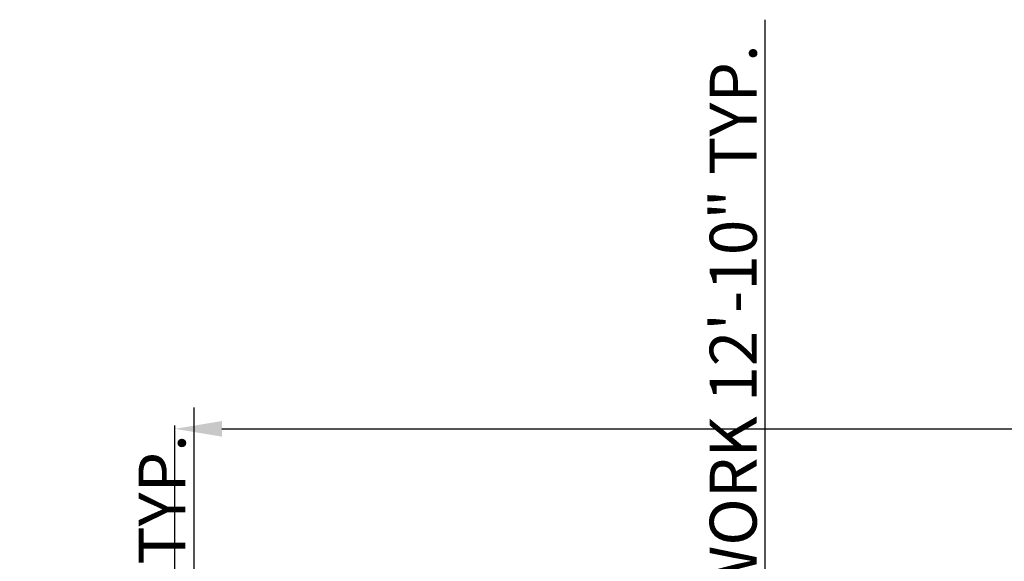
# Model space of a CAD drawing. Units: inches. Extents: x 2043 to 3177, y 1429 to 2563.
# Tile 12 of 14: x 2174 to 2552, y 2355 to 2563. Entities that reach past the tile are written whole.
import ezdxf

# ---------------------------------------------------------------- set-up
doc = ezdxf.new("R2010")
doc.units = ezdxf.units.IN
doc.layers.add('A-ANNO-DIMS', color=2, linetype='Continuous', lineweight=13)
doc.styles.get("Standard").update_dxf_attribs({"font": 'arial.ttf'})
doc.dimstyles.new('ISO-25', dxfattribs={"dimtxt": 18, "dimasz": 18, "dimexe": 1.25, "dimexo": 0.625, "dimtad": 1, "dimlunit": 3, "dimtxsty": 'Standard', "dimcen": 2.5, "dimadec": 0, "dimazin": 0, "dimtfac": 1, "dimtmove": 0, "dimatfit": 3, "dimfxl": 1, "dimarcsym": 0})

# ---------------------------------------------------------------- blocks, each defined once
blk = doc.blocks.new('*D30')
at = {"layer": 'A-ANNO-DIMS', "color": 0, "lineweight": -2, "transparency": 16777216}
for p, q in [((2233.74, 2262.02), (2233.74, 2407.15)), ((2251.74, 2405.9), (2962.74, 2405.9)), ((2980.74, 2262.02), (2980.74, 2407.15))]:
    blk.add_line(p, q, dxfattribs=at)
at = {"layer": 'A-ANNO-DIMS', "color": 0, "transparency": 16777216}
for points in [[(2251.74, 2408.9), (2251.74, 2402.9), (2233.74, 2405.9)], [(2962.74, 2408.9), (2962.74, 2402.9), (2980.74, 2405.9)]]:
    blk.add_solid(points, dxfattribs=at)
at = {"layer": 'Defpoints', "color": 0, "transparency": 16777216}
for p in [(2980.74, 2405.9), (2233.74, 2261.39), (2980.74, 2261.39)]:
    blk.add_point(p, dxfattribs=at)
at = {"layer": 'A-ANNO-DIMS', "color": 0, "transparency": 16777216, "insert": (2607.24, 2415.72), "char_height": 18, "attachment_point": 5}
blk.add_mtext('75\'-0"', dxfattribs=at)
blk = doc.blocks.new('*D59')
at = {"layer": 'A-ANNO-DIMS', "color": 0, "lineweight": -2, "transparency": 16777216}
for p, q in [((2241.04, 2086.9), (2241.04, 2414.07)), ((2243.29, 2068.9), (2239.79, 2068.9)), ((2241.04, 2049.7), (2241.04, 2068.9)), ((2243.29, 2049.7), (2239.79, 2049.7)), ((2241.04, 2031.7), (2241.04, 2013.7))]:
    blk.add_line(p, q, dxfattribs=at)
at = {"layer": 'A-ANNO-DIMS', "color": 0, "transparency": 16777216}
for points in [[(2238.04, 2086.9), (2244.04, 2086.9), (2241.04, 2068.9)], [(2238.04, 2031.7), (2244.04, 2031.7), (2241.04, 2049.7)]]:
    blk.add_solid(points, dxfattribs=at)
at = {"layer": 'Defpoints', "color": 0, "transparency": 16777216}
for p in [(2241.04, 2068.9), (2243.92, 2068.9), (2243.92, 2049.7)]:
    blk.add_point(p, dxfattribs=at)
at = {"layer": 'A-ANNO-DIMS', "color": 0, "transparency": 16777216, "insert": (2231.1, 2259.48), "char_height": 18, "attachment_point": 5, "rotation": 90}
blk.add_mtext('CORNER BASIN 1\'-7" TYP.', dxfattribs=at)
blk = doc.blocks.new('*D63')
at = {"layer": 'A-ANNO-DIMS', "color": 0, "lineweight": -2, "transparency": 16777216}
for p, q in [((2460.06, 2252.39), (2460.06, 2562.81)), ((2437.62, 2252.39), (2461.31, 2252.39)), ((2460.06, 2116.64), (2460.06, 2234.39)), ((2437.62, 2098.64), (2461.31, 2098.64))]:
    blk.add_line(p, q, dxfattribs=at)
at = {"layer": 'A-ANNO-DIMS', "color": 0, "transparency": 16777216}
for points in [[(2457.06, 2234.39), (2463.06, 2234.39), (2460.06, 2252.39)], [(2457.06, 2116.64), (2463.06, 2116.64), (2460.06, 2098.64)]]:
    blk.add_solid(points, dxfattribs=at)
at = {"layer": 'Defpoints', "color": 0, "transparency": 16777216}
for p in [(2436.99, 2252.39), (2460.06, 2252.39), (2436.99, 2098.64)]:
    blk.add_point(p, dxfattribs=at)
at = {"layer": 'A-ANNO-DIMS', "color": 0, "transparency": 16777216, "insert": (2450.12, 2416.6), "char_height": 18, "attachment_point": 5, "rotation": 90}
blk.add_mtext('CASEWORK 12\'-10" TYP.', dxfattribs=at)

msp = doc.modelspace()

# ---------------------------------------------------------------- dimensions: what is measured, and where the dimension line sits
at = {"layer": 'A-ANNO-DIMS'}
for base, p1, p2, text, picture, middle in [((2460.057080565, 2252.39332903), (2436.994580565, 2098.64332903), (2436.994580565, 2252.39332903), 'CASEWORK <> TYP.', '*D63', (2450.118983703, 2416.602230804)), ((2241.039, 2068.902), (2243.919, 2049.702), (2243.919, 2068.902), 'CORNER BASIN <> TYP.', '*D59', (2231.101, 2259.485))]:
    dim = msp.add_linear_dim(base=base, p1=p1, p2=p2, angle=90, text=text, dimstyle='ISO-25', override={"dimdec": 1, "dimlfac": 1, "dimrnd": 0, "dimzin": 1, "dimdsep": 46, "dimlunit": 4, "dimfrac": 2}, dxfattribs=at)
    dim.commit()
    dim.dimension.update_dxf_attribs({"geometry": picture, "text_midpoint": middle})
dim = msp.add_linear_dim(base=(2980.745, 2405.904), p1=(2233.745, 2261.393), p2=(2980.745, 2261.393), text='75\'-0"', dimstyle='ISO-25', override={"dimclrd": 0, "dimclre": 0, "dimclrt": 0}, dxfattribs=at)
dim.commit()
dim.dimension.update_dxf_attribs({"geometry": '*D30', "text_midpoint": (2607.245, 2415.72)})

doc.saveas('drawing.dxf')
